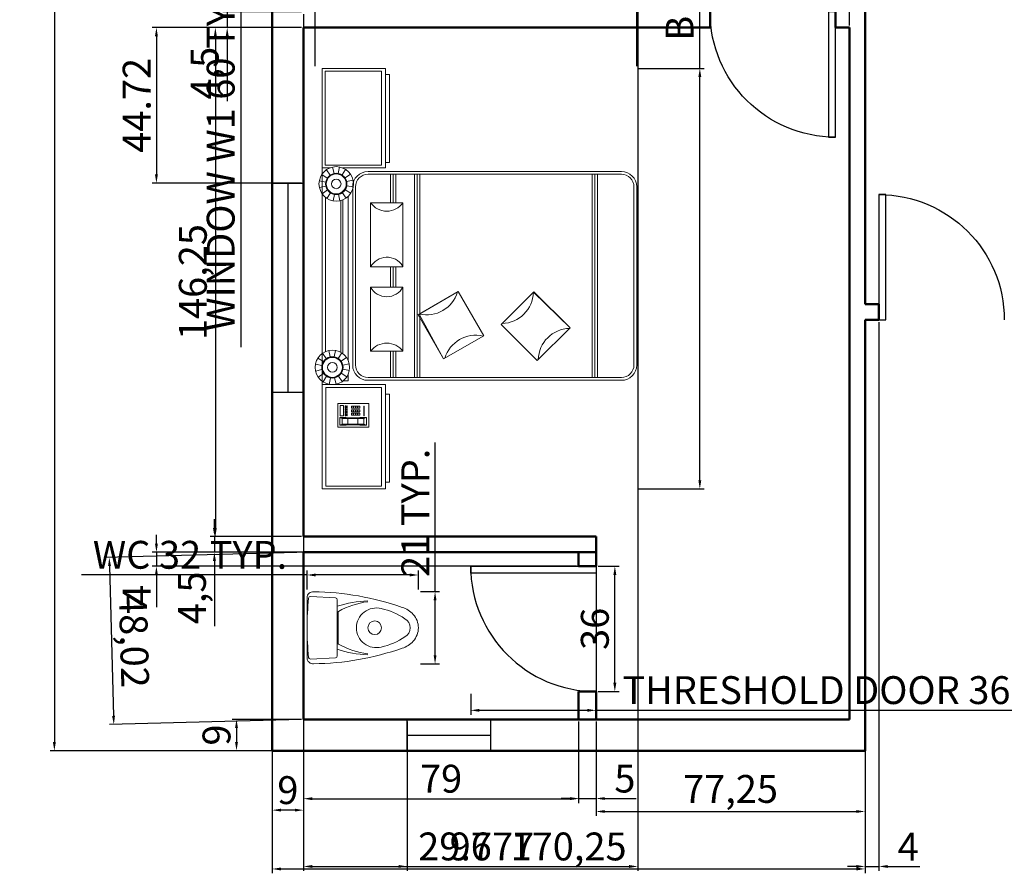
# Model space of a CAD drawing. Units: inches. Extents: x -349 to 9053, y 635 to 6001.
# Tile 2 of 7: x 257 to 540, y 635 to 880. Entities that reach past the tile are written whole.
import ezdxf

# ---------------------------------------------------------------- set-up
doc = ezdxf.new("R2010")
doc.units = ezdxf.units.IN
for name, color, linetype, lineweight in [('A-ANNO-DIMS', 2, 'Continuous', 18), ('A-DOOR', 3, 'Continuous', 25), ('A-FLOR-FIXT', 7, 'Continuous', 18), ('A-FURN', 8, 'Continuous', 18), ('A-GLAZ', 4, 'Continuous', 25), ('A-WALL', 7, 'Continuous', 50)]:
    doc.layers.add(name, color=color, linetype=linetype, lineweight=lineweight)
doc.styles.get("Standard").update_dxf_attribs({"font": 'arial.ttf'})
doc.dimstyles.new('ISO-25', dxfattribs={"dimtxt": 8, "dimasz": 2.5, "dimexe": 1.25, "dimexo": 0.625, "dimtad": 1, "dimtxsty": 'Standard', "dimcen": 2.5, "dimadec": 0, "dimazin": 0, "dimtfac": 1, "dimtmove": 0, "dimatfit": 3, "dimfxl": 1, "dimarcsym": 0})

# ---------------------------------------------------------------- blocks, each defined once
blk = doc.blocks.new('A$C18EB7ED0')
for p, q in [((0.7653, 2.1814), (0.7911, 2.1442)), ((0.8076, 2.1998), (0.8172, 2.1555)), ((0.8537, 2.2006), (0.8456, 2.1559)), ((0.8966, 2.1836), (0.8721, 2.1455)), ((2.0643, 2.1733), (2.0739, 2.129)), ((2.1105, 2.1741), (2.1024, 2.1295)), ((0, 2.1539), (2.8801, 2.1539)), ((0, 1.7209), (0, 2.1539)), ((0.0187, 2.129), (0.695, 2.129)), ((0.0187, 1.7489), (0.0187, 2.129)), ((0.695, 2.129), (0.695, 1.7489)), ((0.7156, 2.1539), (0.7156, 1.7209)), ((0.7162, 2.1054), (0.7608, 2.0973)), ((0.7332, 2.1483), (0.7713, 2.1237)), ((0.9298, 2.1515), (0.8925, 2.1257)), ((0.9481, 2.1092), (0.9038, 2.0996)), ((0.941, 2.1314), (1.9968, 2.1314)), ((1.9899, 2.1218), (2.028, 2.0973)), ((2.022, 2.155), (2.0478, 2.1177)), ((2.1534, 2.1571), (2.1288, 2.119)), ((2.1865, 2.1251), (2.1493, 2.0992)), ((2.1997, 2.1), (2.1997, 2.1539)), ((2.2184, 2.1337), (2.8624, 2.1337)), ((2.2184, 1.7489), (2.2184, 2.1337)), ((2.8624, 2.1337), (2.8624, 1.7489)), ((2.8801, 2.1539), (2.8801, 1.7209)), ((0.5857, 2.0461), (0.4227, 2.0461)), ((0.4227, 2.0461), (0.4227, 1.8353)), ((0.4366, 2.0335), (0.4439, 2.018)), ((0.4903, 2.0335), (0.4366, 2.0335)), ((0.4366, 2.0335), (0.4366, 1.9902)), ((0.4824, 2.018), (0.4903, 2.0335)), ((0.4903, 1.9902), (0.4903, 2.0338)), ((0.5706, 2.0307), (0.4996, 2.0307)), ((0.4996, 2.0307), (0.4996, 2.0082)), ((0.5706, 2.0082), (0.5706, 2.0307)), ((0.5857, 1.8353), (0.5857, 2.0461)), ((0.717, 2.0593), (0.7613, 2.0688)), ((0.7353, 2.0169), (0.7726, 2.0427)), ((0.7685, 1.9849), (0.7931, 2.023)), ((0.8999, 1.987), (0.8741, 2.0243)), ((0.9319, 2.0202), (0.8938, 2.0447)), ((0.9489, 2.0631), (0.9043, 2.0712)), ((1.9752, 2.0268), (0.9359, 2.0268)), ((1.973, 2.0789), (2.0176, 2.0708)), ((1.9737, 2.0328), (2.0181, 2.0424)), ((2.2049, 2.0827), (2.1606, 2.0731)), ((2.2056, 2.0366), (2.161, 2.0447)), ((0.4366, 1.9902), (0.4391, 1.9789)), ((0.4391, 1.9789), (0.4391, 1.9067)), ((0.4824, 2.018), (0.4439, 2.018)), ((0.4824, 2.018), (0.4439, 2.018)), ((0.4439, 2.018), (0.4439, 1.8697)), ((0.4824, 1.978), (0.4439, 1.978)), ((0.4824, 1.8697), (0.4824, 2.018)), ((0.4903, 1.9902), (0.4871, 1.9789)), ((0.4871, 1.9789), (0.4871, 1.908)), ((0.4996, 2.0082), (0.5706, 2.0082)), ((0.514, 1.9963), (0.5013, 1.9963)), ((0.5013, 1.9963), (0.5013, 1.992)), ((0.5013, 1.992), (0.514, 1.992)), ((0.514, 1.9864), (0.5013, 1.9864)), ((0.5013, 1.9864), (0.5013, 1.9821)), ((0.5013, 1.9821), (0.514, 1.9821)), ((0.514, 1.992), (0.514, 1.9963)), ((0.514, 1.9821), (0.514, 1.9864)), ((0.5324, 1.9963), (0.5196, 1.9963)), ((0.5196, 1.9963), (0.5196, 1.992)), ((0.5196, 1.992), (0.5324, 1.992)), ((0.5324, 1.9864), (0.5196, 1.9864)), ((0.5196, 1.9864), (0.5196, 1.9821)), ((0.5196, 1.9821), (0.5324, 1.9821)), ((0.5324, 1.992), (0.5324, 1.9963)), ((0.5324, 1.9821), (0.5324, 1.9864)), ((0.5507, 1.9963), (0.538, 1.9963)), ((0.538, 1.9963), (0.538, 1.992)), ((0.538, 1.992), (0.5507, 1.992)), ((0.5507, 1.9864), (0.538, 1.9864)), ((0.538, 1.9864), (0.538, 1.9821)), ((0.538, 1.9821), (0.5507, 1.9821)), ((0.5507, 1.992), (0.5507, 1.9963)), ((0.5507, 1.9821), (0.5507, 1.9864)), ((0.5691, 1.9963), (0.5564, 1.9963)), ((0.5564, 1.9963), (0.5564, 1.992)), ((0.5564, 1.992), (0.5691, 1.992)), ((0.5691, 1.9864), (0.5564, 1.9864)), ((0.5564, 1.9864), (0.5564, 1.9821)), ((0.5564, 1.9821), (0.5691, 1.9821)), ((0.5691, 1.992), (0.5691, 1.9963)), ((0.5691, 1.9821), (0.5691, 1.9864)), ((0.7411, 2.0132), (0.7411, 1.9754)), ((0.7411, 1.9754), (0.7863, 1.9754)), ((0.8114, 1.9679), (0.8195, 2.0125)), ((0.8575, 1.9687), (0.848, 2.013)), ((0.8788, 1.9754), (2.0045, 1.9754)), ((1.9798, 2.0132), (0.9271, 2.0132)), ((1.9921, 1.9905), (2.0294, 2.0163)), ((2.0252, 1.9584), (2.0498, 1.9965)), ((2.0682, 1.9414), (2.0763, 1.986)), ((2.1143, 1.9422), (2.1047, 1.9865)), ((2.1566, 1.9605), (2.1308, 1.9978)), ((2.1887, 1.9937), (2.1506, 2.0183)), ((2.1742, 1.9754), (2.1771, 1.9754)), ((2.1771, 1.9754), (2.1771, 1.9785)), ((2.1997, 1.7209), (2.1997, 2.0155)), ((0.4391, 1.9067), (0.4366, 1.8971)), ((0.4366, 1.8971), (0.4366, 1.8504)), ((0.4439, 1.9101), (0.4824, 1.9101)), ((0.4871, 1.908), (0.4903, 1.8971)), ((0.4903, 1.8499), (0.4903, 1.8971)), ((0.52, 1.9534), (0.5062, 1.9534)), ((0.5062, 1.9534), (0.5062, 1.9417)), ((0.5062, 1.9417), (0.52, 1.9417)), ((0.52, 1.9385), (0.5062, 1.9385)), ((0.5062, 1.9385), (0.5062, 1.9269)), ((0.5062, 1.9269), (0.52, 1.9269)), ((0.52, 1.9237), (0.5062, 1.9237)), ((0.5062, 1.9237), (0.5062, 1.9121)), ((0.5062, 1.9121), (0.52, 1.9121)), ((0.52, 1.9089), (0.5062, 1.9089)), ((0.5062, 1.9089), (0.5062, 1.8972)), ((0.5062, 1.8972), (0.52, 1.8972)), ((0.52, 1.9417), (0.52, 1.9534)), ((0.52, 1.9269), (0.52, 1.9385)), ((0.52, 1.9121), (0.52, 1.9237)), ((0.52, 1.8972), (0.52, 1.9089)), ((0.5426, 1.9534), (0.5288, 1.9534)), ((0.5288, 1.9534), (0.5288, 1.9417)), ((0.5288, 1.9417), (0.5426, 1.9417)), ((0.5426, 1.9385), (0.5288, 1.9385)), ((0.5288, 1.9385), (0.5288, 1.9269)), ((0.5288, 1.9269), (0.5426, 1.9269)), ((0.5426, 1.9237), (0.5288, 1.9237)), ((0.5288, 1.9237), (0.5288, 1.9121)), ((0.5288, 1.9121), (0.5426, 1.9121)), ((0.5426, 1.9089), (0.5288, 1.9089)), ((0.5288, 1.9089), (0.5288, 1.8972)), ((0.5288, 1.8972), (0.5426, 1.8972)), ((0.5426, 1.9417), (0.5426, 1.9534)), ((0.5426, 1.9269), (0.5426, 1.9385)), ((0.5426, 1.9121), (0.5426, 1.9237)), ((0.5426, 1.8972), (0.5426, 1.9089)), ((0.5659, 1.9534), (0.5521, 1.9534)), ((0.5521, 1.9534), (0.5521, 1.9417)), ((0.5521, 1.9417), (0.5659, 1.9417)), ((0.5659, 1.9385), (0.5521, 1.9385)), ((0.5521, 1.9385), (0.5521, 1.9269)), ((0.5521, 1.9269), (0.5659, 1.9269)), ((0.5659, 1.9237), (0.5521, 1.9237)), ((0.5521, 1.9237), (0.5521, 1.9121)), ((0.5521, 1.9121), (0.5659, 1.9121)), ((0.5659, 1.9089), (0.5521, 1.9089)), ((0.5521, 1.9089), (0.5521, 1.8972)), ((0.5521, 1.8972), (0.5659, 1.8972)), ((0.5659, 1.9417), (0.5659, 1.9534)), ((0.5659, 1.9269), (0.5659, 1.9385)), ((0.5659, 1.9121), (0.5659, 1.9237)), ((0.5659, 1.8972), (0.5659, 1.9089)), ((2.0691, 1.9452), (0.8491, 1.9452)), ((2.0691, 1.926), (0.8491, 1.926)), ((0.4227, 1.8353), (0.5857, 1.8353)), ((0.4439, 1.8697), (0.4366, 1.8504)), ((0.4366, 1.8504), (0.4903, 1.8504)), ((0.4824, 1.8697), (0.4439, 1.8697)), ((0.4439, 1.8697), (0.4824, 1.8697)), ((0.4903, 1.8504), (0.4824, 1.8697)), ((0.5208, 1.8697), (0.5009, 1.8697)), ((0.5009, 1.8697), (0.5009, 1.8657)), ((0.5009, 1.8657), (0.5208, 1.8657)), ((0.5208, 1.8657), (0.5208, 1.8697)), ((0.5433, 1.8697), (0.5234, 1.8697)), ((0.5234, 1.8697), (0.5234, 1.8657)), ((0.5234, 1.8657), (0.5433, 1.8657)), ((0.5433, 1.8657), (0.5433, 1.8697)), ((0.5658, 1.8697), (0.546, 1.8697)), ((0.546, 1.8697), (0.546, 1.8657)), ((0.546, 1.8657), (0.5658, 1.8657)), ((0.5658, 1.8657), (0.5658, 1.8697)), ((0.7439, 1.8401), (0.7439, 0.1052)), ((0.7632, 1.8401), (0.7632, 0.1052)), ((0.9429, 1.8231), (1.3829, 1.8231)), ((0.9429, 1.601), (0.9429, 1.8231)), ((1.3829, 1.8231), (1.3829, 1.601)), ((1.5207, 1.601), (1.5207, 1.8231)), ((1.5207, 1.8231), (1.9608, 1.8231)), ((1.9608, 1.8231), (1.9608, 1.601)), ((2.155, 0.1052), (2.155, 1.8401)), ((2.1743, 0.1052), (2.1743, 1.8401)), ((0.7156, 1.7209), (0, 1.7209)), ((0, 1.7209), (0.6483, 1.7209)), ((0.695, 1.7489), (0.0187, 1.7489)), ((0.0462, 1.6929), (0.0462, 1.7209)), ((0.6483, 1.6929), (0.0462, 1.6929)), ((0.6483, 1.7209), (0.6483, 1.6929)), ((0.7632, 1.6858), (0.9429, 1.6858)), ((1.3829, 1.6858), (1.5207, 1.6858)), ((1.9608, 1.6858), (2.155, 1.6858)), ((2.8801, 1.7209), (2.1997, 1.7209)), ((2.8624, 1.7489), (2.2184, 1.7489)), ((2.2369, 1.7209), (2.8801, 1.7209)), ((2.2369, 1.6929), (2.2369, 1.7209)), ((2.839, 1.6929), (2.2369, 1.6929)), ((2.839, 1.7209), (2.839, 1.6929)), ((0.7632, 1.6678), (0.9429, 1.6678)), ((0.7632, 1.6498), (0.9429, 1.6498)), ((1.3829, 1.6678), (1.5207, 1.6678)), ((1.3829, 1.6498), (1.5207, 1.6498)), ((1.9608, 1.6678), (2.155, 1.6678)), ((1.9608, 1.6498), (2.155, 1.6498)), ((1.3829, 1.601), (0.9429, 1.601)), ((1.9608, 1.601), (1.5207, 1.601)), ((0.7632, 1.5215), (2.155, 1.5215)), ((0.7632, 1.5035), (2.155, 1.5035)), ((0.7632, 1.4855), (2.155, 1.4855)), ((0.8904, 1.3226), (1.1935, 1.4976)), ((0.8904, 1.3226), (1.1982, 1.4894)), ((1.1935, 1.4976), (1.3524, 1.2224)), ((1.1982, 1.4894), (1.3524, 1.2224)), ((1.0493, 1.0474), (0.8904, 1.3226)), ((1.0493, 1.0474), (0.8904, 1.3226)), ((1.3524, 1.2224), (1.0493, 1.0474)), ((1.3524, 1.2224), (1.0493, 1.0474)), ((0.8789, 0.6811), (1.1264, 0.9286)), ((0.8789, 0.6811), (1.1264, 0.9286)), ((1.1264, 0.9286), (1.3473, 0.7077)), ((1.1264, 0.9286), (1.3511, 0.7039)), ((1.1036, 0.4564), (0.8789, 0.6811)), ((1.1036, 0.4564), (0.8789, 0.6811)), ((1.3473, 0.7077), (1.1036, 0.4564)), ((1.3511, 0.7039), (1.1036, 0.4564)), ((0.7632, 0.3045), (2.155, 0.3045)), ((0.7632, 0.2865), (2.155, 0.2865)), ((0.7632, 0.2685), (2.155, 0.2685)), ((0.8491, 0.0193), (2.0691, 0.0193)), ((0.8491, 0), (2.0691, 0))]:
    blk.add_line(p, q)
for centre, radius in [((0.8326, 2.0842), 0.1182), ((2.0893, 2.0578), 0.1182), ((0.8326, 2.0842), 0.0729), ((0.8326, 2.0842), 0.0684), ((0.8326, 2.0842), 0.0328), ((2.0893, 2.0578), 0.0729), ((2.0893, 2.0578), 0.0684), ((2.0893, 2.0578), 0.0328)]:
    blk.add_circle(centre, radius)
for centre, radius, start, end in [((0.8491, 1.8401), 0.1052, 90, 180), ((0.8491, 1.8401), 0.0859, 90, 180), ((2.0691, 1.8401), 0.1052, 0, 90), ((2.0691, 1.8401), 0.0859, 0, 90), ((0.8604, 1.712), 0.1383, 306.59595, 53.40405), ((1.4431, 1.712), 0.1263, 118.46186, 241.53814), ((1.4584, 1.7106), 0.1286, 303.40233, 61.02638), ((2.0371, 1.712), 0.1347, 124.50267, 235.49733), ((1.4126, 1.4383), 0.2204, 166.58792, 253.41208), ((0.8322, 1.1031), 0.2204, 346.58792, 73.41208), ((1.3534, 0.928), 0.2204, 181.58792, 268.41208), ((0.8795, 0.4541), 0.2204, 1.58792, 88.41208), ((0.8491, 0.1052), 0.1052, 180, 270), ((0.8491, 0.1052), 0.0859, 180, 270), ((2.0691, 0.1052), 0.1052, 270, 0), ((2.0691, 0.1052), 0.0859, 270, 0)]:
    blk.add_arc(centre, radius, start, end)
blk = doc.blocks.new('A$C444A5E9C')
at = {"ltscale": 20}
for p, q in [((0.2458, 0.76), (0.0398, 0.76)), ((0.0411, 0.5655), (0.0321, 0.7371)), ((0.0536, 0.5537), (0.2458, 0.5537)), ((0.141, 0.5487), (0.2458, 0.5487))]:
    blk.add_line(p, q, dxfattribs=at)
for p, q in [((0.2458, 0.76), (0.4517, 0.76)), ((0.4504, 0.5655), (0.4594, 0.7371)), ((0.4379, 0.5537), (0.2458, 0.5537)), ((0.3505, 0.5487), (0.2458, 0.5487))]:
    blk.add_line(p, q)
blk.add_circle((0.2458, 0.2982), 0.0465, dxfattribs=at)
for centre, radius, start, end in [((0.0398, 0.72), 0.04, 90, 185.821), ((0.0441, 0.7377), 0.012, 95.84387, 183), ((0.2455, -1.2297), 1.9897, 89.99241, 95.84387), ((1.8697, 0.7335), 1.8698, 180.53729, 199.44062), ((0.0536, 0.5662), 0.0125, 183, 270), ((0.7661, 0.3277), 0.7045, 161.29061, 178.53633), ((0.58, 0.2848), 0.5159, 149.71646, 173.22437), ((0.141, 0.5412), 0.0075, 90, 149.71646), ((0.2463, 0.2875), 0.1361, 90.23685, 194.54903), ((0.2452, 0.2875), 0.1361, 345.45097, 89.76315), ((0.561, 0.3494), 0.4566, 192.1399, 214.27057), ((-0.0695, 0.3494), 0.4566, 325.72943, 347.8601), ((0.2665, 0.1585), 0.1669, 196.47232, 227.66237), ((0.2465, 0.1287), 0.0727, 210.08399, 269.41891), ((0.245, 0.1287), 0.0727, 270.58109, 329.91601), ((0.2458, 0.137), 0.137, 228.04012, 270)]:
    blk.add_arc(centre, radius, start, end, dxfattribs=at)
for centre, radius, start, end in [((0.246, -1.2297), 1.9897, 84.15613, 90.00759), ((0.4474, 0.7377), 0.012, 357, 84.15613), ((0.4517, 0.72), 0.04, 354.179, 90), ((-1.3782, 0.7335), 1.8698, 340.55938, 359.46271), ((0.3505, 0.5412), 0.0075, 30.28354, 90), ((-0.0885, 0.2848), 0.5159, 6.77563, 30.28354), ((-0.2746, 0.3277), 0.7045, 1.46367, 18.70939), ((0.4379, 0.5662), 0.0125, 270, 357), ((0.225, 0.1585), 0.1669, 312.33763, 343.52768), ((0.2458, 0.137), 0.137, 270, 311.95988)]:
    blk.add_arc(centre, radius, start, end)
blk = doc.blocks.new('*D20')
at = {"layer": 'A-ANNO-DIMS', "color": 0, "lineweight": -2, "transparency": 16777216}
for p, q in [((317.08, 884.75), (317.08, 887.25)), ((338.38, 882.25), (315.83, 882.25)), ((317.08, 882.25), (317.08, 877.75)), ((338.38, 877.75), (315.83, 877.75)), ((317.08, 875.25), (317.08, 856.55))]:
    blk.add_line(p, q, dxfattribs=at)
at = {"layer": 'A-ANNO-DIMS', "color": 0, "transparency": 16777216}
for points in [[(316.66, 884.75), (317.5, 884.75), (317.08, 882.25)], [(316.66, 875.25), (317.5, 875.25), (317.08, 877.75)]]:
    blk.add_solid(points, dxfattribs=at)
at = {"layer": 'Defpoints', "color": 0, "transparency": 16777216}
for p in [(339, 882.25), (317.08, 877.75), (339, 877.75)]:
    blk.add_point(p, dxfattribs=at)
at = {"layer": 'A-ANNO-DIMS', "color": 0, "transparency": 16777216, "insert": (311.66, 864.65), "char_height": 8, "attachment_point": 5, "rotation": 90}
blk.add_mtext('4,5', dxfattribs=at)
blk = doc.blocks.new('*D21')
at = {"layer": 'A-ANNO-DIMS', "color": 0, "lineweight": -2, "transparency": 16777216}
for p, q in [((338.38, 877.75), (312.42, 877.75)), ((313.67, 875.25), (313.67, 734)), ((338.38, 731.5), (312.42, 731.5))]:
    blk.add_line(p, q, dxfattribs=at)
at = {"layer": 'A-ANNO-DIMS', "color": 0, "transparency": 16777216}
for points in [[(313.26, 875.25), (314.09, 875.25), (313.67, 877.75)], [(313.26, 734), (314.09, 734), (313.67, 731.5)]]:
    blk.add_solid(points, dxfattribs=at)
at = {"layer": 'Defpoints', "color": 0, "transparency": 16777216}
for p in [(339, 877.75), (313.67, 731.5), (339, 731.5)]:
    blk.add_point(p, dxfattribs=at)
at = {"layer": 'A-ANNO-DIMS', "color": 0, "transparency": 16777216, "insert": (308.24, 804.62), "char_height": 8, "attachment_point": 5, "rotation": 90}
blk.add_mtext('146,25', dxfattribs=at)
blk = doc.blocks.new('*D22')
at = {"layer": 'A-ANNO-DIMS', "color": 0, "lineweight": -2, "transparency": 16777216}
for p, q in [((313.4, 734), (313.4, 736.5)), ((338.38, 731.5), (312.15, 731.5)), ((313.4, 731.5), (313.4, 727)), ((338.38, 727), (312.15, 727)), ((313.4, 724.5), (313.4, 705.8))]:
    blk.add_line(p, q, dxfattribs=at)
at = {"layer": 'A-ANNO-DIMS', "color": 0, "transparency": 16777216}
for points in [[(312.99, 734), (313.82, 734), (313.4, 731.5)], [(312.99, 724.5), (313.82, 724.5), (313.4, 727)]]:
    blk.add_solid(points, dxfattribs=at)
at = {"layer": 'Defpoints', "color": 0, "transparency": 16777216}
for p in [(339, 731.5), (313.4, 727), (339, 727)]:
    blk.add_point(p, dxfattribs=at)
at = {"layer": 'A-ANNO-DIMS', "color": 0, "transparency": 16777216, "insert": (307.99, 713.9), "char_height": 8, "attachment_point": 5, "rotation": 90}
blk.add_mtext('4,5', dxfattribs=at)
blk = doc.blocks.new('*D23')
at = {"layer": 'A-ANNO-DIMS', "color": 0, "lineweight": -2, "transparency": 16777216}
for p, q in [((337.08, 726.98), (281.96, 725.49)), ((283.28, 723.03), (284.44, 680.02)), ((338.38, 678.98), (283.26, 677.49))]:
    blk.add_line(p, q, dxfattribs=at)
at = {"layer": 'A-ANNO-DIMS', "color": 0, "transparency": 16777216}
for points in [[(283.69, 723.04), (282.86, 723.02), (283.21, 725.53)], [(284.86, 680.04), (284.02, 680.01), (284.51, 677.53)]]:
    blk.add_solid(points, dxfattribs=at)
at = {"layer": 'Defpoints', "color": 0, "transparency": 16777216}
for p in [(337.7, 727), (339, 679), (284.51, 677.53)]:
    blk.add_point(p, dxfattribs=at)
at = {"layer": 'A-ANNO-DIMS', "color": 0, "transparency": 16777216, "insert": (289.29, 701.67), "char_height": 8, "attachment_point": 5, "rotation": 271.5498}
blk.add_mtext('48,02', dxfattribs=at)
blk = doc.blocks.new('*D24')
at = {"layer": 'A-ANNO-DIMS', "color": 0, "lineweight": -2, "transparency": 16777216}
for p, q in [((338.38, 679), (318.49, 679)), ((319.74, 676.5), (319.74, 672.5)), ((338.38, 670), (318.49, 670))]:
    blk.add_line(p, q, dxfattribs=at)
at = {"layer": 'A-ANNO-DIMS', "color": 0, "transparency": 16777216}
for points in [[(319.33, 676.5), (320.16, 676.5), (319.74, 679)], [(319.33, 672.5), (320.16, 672.5), (319.74, 670)]]:
    blk.add_solid(points, dxfattribs=at)
at = {"layer": 'Defpoints', "color": 0, "transparency": 16777216}
for p in [(339, 679), (319.74, 670), (339, 670)]:
    blk.add_point(p, dxfattribs=at)
at = {"layer": 'A-ANNO-DIMS', "color": 0, "transparency": 16777216, "insert": (315.04, 674.5), "char_height": 8, "attachment_point": 5, "rotation": 90}
blk.add_mtext('9', dxfattribs=at)
blk = doc.blocks.new('*D25')
at = {"layer": 'A-ANNO-DIMS', "color": 0, "lineweight": -2, "transparency": 16777216}
for p, q in [((330, 678.38), (330, 651.68)), ((339, 678.38), (339, 651.68)), ((336.5, 652.93), (332.5, 652.93))]:
    blk.add_line(p, q, dxfattribs=at)
at = {"layer": 'A-ANNO-DIMS', "color": 0, "transparency": 16777216}
for points in [[(332.5, 653.35), (332.5, 652.52), (330, 652.93)], [(336.5, 653.35), (336.5, 652.52), (339, 652.93)]]:
    blk.add_solid(points, dxfattribs=at)
at = {"layer": 'Defpoints', "color": 0, "transparency": 16777216}
for p in [(330, 679), (339, 679), (330, 652.93)]:
    blk.add_point(p, dxfattribs=at)
at = {"layer": 'A-ANNO-DIMS', "color": 0, "transparency": 16777216, "insert": (334.5, 657.64), "char_height": 8, "attachment_point": 5}
blk.add_mtext('9', dxfattribs=at)
blk = doc.blocks.new('*D26')
at = {"layer": 'A-ANNO-DIMS', "color": 0, "lineweight": -2, "transparency": 16777216}
for p, q in [((339, 678.38), (339, 654.96)), ((418, 678.38), (418, 654.96)), ((341.5, 656.21), (415.5, 656.21))]:
    blk.add_line(p, q, dxfattribs=at)
at = {"layer": 'A-ANNO-DIMS', "color": 0, "transparency": 16777216}
for points in [[(341.5, 656.63), (341.5, 655.8), (339, 656.21)], [(415.5, 656.63), (415.5, 655.8), (418, 656.21)]]:
    blk.add_solid(points, dxfattribs=at)
at = {"layer": 'Defpoints', "color": 0, "transparency": 16777216}
for p in [(339, 679), (418, 679), (418, 656.21)]:
    blk.add_point(p, dxfattribs=at)
at = {"layer": 'A-ANNO-DIMS', "color": 0, "transparency": 16777216, "insert": (378.5, 660.92), "char_height": 8, "attachment_point": 5}
blk.add_mtext('79', dxfattribs=at)
blk = doc.blocks.new('*D27')
at = {"layer": 'A-ANNO-DIMS', "color": 0, "lineweight": -2, "transparency": 16777216}
for p, q in [((418, 678.38), (418, 655.02)), ((423, 678.38), (423, 655.02)), ((415.5, 656.27), (413, 656.27)), ((418, 656.27), (423, 656.27)), ((425.5, 656.27), (434.55, 656.27))]:
    blk.add_line(p, q, dxfattribs=at)
at = {"layer": 'A-ANNO-DIMS', "color": 0, "transparency": 16777216}
for points in [[(415.5, 656.68), (415.5, 655.85), (418, 656.27)], [(425.5, 656.68), (425.5, 655.85), (423, 656.27)]]:
    blk.add_solid(points, dxfattribs=at)
at = {"layer": 'Defpoints', "color": 0, "transparency": 16777216}
for p in [(418, 679), (423, 679), (423, 656.27)]:
    blk.add_point(p, dxfattribs=at)
at = {"layer": 'A-ANNO-DIMS', "color": 0, "transparency": 16777216, "insert": (431.28, 660.96), "char_height": 8, "attachment_point": 5}
blk.add_mtext('5', dxfattribs=at)
blk = doc.blocks.new('*D28')
at = {"layer": 'A-ANNO-DIMS', "color": 0, "lineweight": -2, "transparency": 16777216}
for p, q in [((423, 678.38), (423, 651.29)), ((500.25, 678.38), (500.25, 651.29)), ((425.5, 652.54), (497.75, 652.54))]:
    blk.add_line(p, q, dxfattribs=at)
at = {"layer": 'A-ANNO-DIMS', "color": 0, "transparency": 16777216}
for points in [[(425.5, 652.96), (425.5, 652.13), (423, 652.54)], [(497.75, 652.96), (497.75, 652.13), (500.25, 652.54)]]:
    blk.add_solid(points, dxfattribs=at)
at = {"layer": 'Defpoints', "color": 0, "transparency": 16777216}
for p in [(423, 679), (500.25, 679), (500.25, 652.54)]:
    blk.add_point(p, dxfattribs=at)
at = {"layer": 'A-ANNO-DIMS', "color": 0, "transparency": 16777216, "insert": (461.62, 657.98), "char_height": 8, "attachment_point": 5}
blk.add_mtext('77,25', dxfattribs=at)
blk = doc.blocks.new('*D29')
at = {"layer": 'A-ANNO-DIMS', "color": 0, "lineweight": -2, "transparency": 16777216}
for p, q in [((330, 669.38), (330, 634.78)), ((500.25, 669.38), (500.25, 634.78)), ((332.5, 636.03), (497.75, 636.03))]:
    blk.add_line(p, q, dxfattribs=at)
at = {"layer": 'A-ANNO-DIMS', "color": 0, "transparency": 16777216}
for points in [[(332.5, 636.45), (332.5, 635.61), (330, 636.03)], [(497.75, 636.45), (497.75, 635.61), (500.25, 636.03)]]:
    blk.add_solid(points, dxfattribs=at)
at = {"layer": 'Defpoints', "color": 0, "transparency": 16777216}
for p in [(330, 670), (500.25, 670), (500.25, 636.03)]:
    blk.add_point(p, dxfattribs=at)
at = {"layer": 'A-ANNO-DIMS', "color": 0, "transparency": 16777216, "insert": (415.12, 641.46), "char_height": 8, "attachment_point": 5}
blk.add_mtext('170,25', dxfattribs=at)
blk = doc.blocks.new('*D31')
at = {"layer": 'A-ANNO-DIMS', "color": 0, "lineweight": -2, "transparency": 16777216}
for p, q in [((338.38, 1126), (266.19, 1126)), ((267.44, 1123.5), (267.44, 672.5)), ((338.38, 670), (266.19, 670))]:
    blk.add_line(p, q, dxfattribs=at)
at = {"layer": 'A-ANNO-DIMS', "color": 0, "transparency": 16777216}
for points in [[(267.02, 1123.5), (267.86, 1123.5), (267.44, 1126)], [(267.02, 672.5), (267.86, 672.5), (267.44, 670)]]:
    blk.add_solid(points, dxfattribs=at)
at = {"layer": 'Defpoints', "color": 0, "transparency": 16777216}
for p in [(339, 1126), (267.44, 670), (339, 670)]:
    blk.add_point(p, dxfattribs=at)
at = {"layer": 'A-ANNO-DIMS', "color": 0, "transparency": 16777216, "insert": (262.73, 898), "char_height": 8, "attachment_point": 5, "rotation": 90}
blk.add_mtext('456', dxfattribs=at)
blk = doc.blocks.new('DOOR-36IN-SWING-WITH-THRESHOLD')
blk.add_line((0, 0), (0, -36))
blk.add_lwpolyline([(-36, 0), (0, 0), (0, -2), (-36, -2)], close=True)
blk.add_arc((0, 0), 36, 180, 270)
blk = doc.blocks.new('DOOR-36IN-SWING')
blk.add_line((0, 0), (-2, 0))
blk.add_lwpolyline([(0, 36), (0, 0), (-2, 0), (-2, 36)], close=True)
blk.add_arc((0, 0), 36, 90, 180)
blk = doc.blocks.new('WIN-60IN')
for p, q in [((0, -4.5), (0, 4.5)), ((60, -4.5), (60, 4.5)), ((0, 0), (60, 0))]:
    blk.add_line(p, q)
blk = doc.blocks.new('WIN-24IN')
for p, q in [((0, -4.5), (0, 4.5)), ((24, -4.5), (24, 4.5)), ((0, 0), (24, 0))]:
    blk.add_line(p, q)
blk = doc.blocks.new('*D41')
at = {"layer": 'A-ANNO-DIMS', "color": 0, "lineweight": -2, "transparency": 16777216}
for p, q in [((387, 686.37), (387, 680.35)), ((423, 686.37), (423, 680.35)), ((389.5, 681.6), (420.5, 681.6)), ((423, 681.6), (547.07, 681.6))]:
    blk.add_line(p, q, dxfattribs=at)
at = {"layer": 'A-ANNO-DIMS', "color": 0, "transparency": 16777216}
for points in [[(389.5, 682.02), (389.5, 681.18), (387, 681.6)], [(420.5, 682.02), (420.5, 681.18), (423, 681.6)]]:
    blk.add_solid(points, dxfattribs=at)
at = {"layer": 'Defpoints', "color": 0, "transparency": 16777216}
for p in [(387, 687), (423, 687), (423, 681.6)]:
    blk.add_point(p, dxfattribs=at)
at = {"layer": 'A-ANNO-DIMS', "color": 0, "transparency": 16777216, "insert": (486.29, 686.37), "char_height": 8, "attachment_point": 5}
blk.add_mtext('THRESHOLD DOOR 36', dxfattribs=at)
blk = doc.blocks.new('*D42')
at = {"layer": 'A-ANNO-DIMS', "color": 0, "lineweight": -2, "transparency": 16777216}
for p, q in [((423.63, 723), (429.65, 723)), ((428.4, 689.5), (428.4, 720.5)), ((423.63, 687), (429.65, 687))]:
    blk.add_line(p, q, dxfattribs=at)
at = {"layer": 'A-ANNO-DIMS', "color": 0, "transparency": 16777216}
for points in [[(427.98, 720.5), (428.82, 720.5), (428.4, 723)], [(427.98, 689.5), (428.82, 689.5), (428.4, 687)]]:
    blk.add_solid(points, dxfattribs=at)
at = {"layer": 'Defpoints', "color": 0, "transparency": 16777216}
for p in [(423, 723), (428.4, 723), (423, 687)]:
    blk.add_point(p, dxfattribs=at)
at = {"layer": 'A-ANNO-DIMS', "color": 0, "transparency": 16777216, "insert": (423.69, 705), "char_height": 8, "attachment_point": 5, "rotation": 90}
blk.add_mtext('36', dxfattribs=at)
blk = doc.blocks.new('*D45')
at = {"layer": 'A-ANNO-DIMS', "color": 0, "lineweight": -2, "transparency": 16777216}
for p, q in [((329.38, 961), (319.75, 961)), ((321, 958.5), (321, 903.5)), ((329.38, 901), (319.75, 901)), ((321, 901), (321, 785.97))]:
    blk.add_line(p, q, dxfattribs=at)
at = {"layer": 'A-ANNO-DIMS', "color": 0, "transparency": 16777216}
for points in [[(320.58, 958.5), (321.42, 958.5), (321, 961)], [(320.58, 903.5), (321.42, 903.5), (321, 901)]]:
    blk.add_solid(points, dxfattribs=at)
at = {"layer": 'Defpoints', "color": 0, "transparency": 16777216}
for p in [(330, 961), (321, 901), (330, 901)]:
    blk.add_point(p, dxfattribs=at)
at = {"layer": 'A-ANNO-DIMS', "color": 0, "transparency": 16777216, "insert": (316.24, 842.24), "char_height": 8, "attachment_point": 5, "rotation": 90}
blk.add_mtext('WINDOW W1 60 TYP.', dxfattribs=at)
blk = doc.blocks.new('*D49')
at = {"layer": 'A-ANNO-DIMS', "color": 0, "lineweight": -2, "transparency": 16777216}
for p, q in [((452.81, 865.99), (452.81, 995.27)), ((435.32, 865.99), (454.06, 865.99)), ((452.81, 747.7), (452.81, 863.49)), ((435.32, 745.2), (454.06, 745.2))]:
    blk.add_line(p, q, dxfattribs=at)
at = {"layer": 'A-ANNO-DIMS', "color": 0, "transparency": 16777216}
for points in [[(452.39, 863.49), (453.23, 863.49), (452.81, 865.99)], [(452.39, 747.7), (453.23, 747.7), (452.81, 745.2)]]:
    blk.add_solid(points, dxfattribs=at)
at = {"layer": 'Defpoints', "color": 0, "transparency": 16777216}
for p in [(434.69, 865.99), (452.81, 865.99), (434.69, 745.2)]:
    blk.add_point(p, dxfattribs=at)
at = {"layer": 'A-ANNO-DIMS', "color": 0, "transparency": 16777216, "insert": (448.04, 931.88), "char_height": 8, "attachment_point": 5, "rotation": 90}
blk.add_mtext('BED GROUP B 121 TYP.', dxfattribs=at)
blk = doc.blocks.new('*D50')
at = {"layer": 'A-ANNO-DIMS', "color": 0, "lineweight": -2, "transparency": 16777216}
for p, q in [((342.32, 866.61), (342.32, 885.35)), ((434.69, 866.61), (434.69, 885.35)), ((432.19, 884.1), (344.82, 884.1))]:
    blk.add_line(p, q, dxfattribs=at)
at = {"layer": 'A-ANNO-DIMS', "color": 0, "transparency": 16777216}
for points in [[(344.82, 884.52), (344.82, 883.69), (342.32, 884.1)], [(432.19, 884.52), (432.19, 883.69), (434.69, 884.1)]]:
    blk.add_solid(points, dxfattribs=at)
at = {"layer": 'Defpoints', "color": 0, "transparency": 16777216}
for p in [(342.32, 884.1), (342.32, 865.99), (434.69, 865.99)]:
    blk.add_point(p, dxfattribs=at)
at = {"layer": 'A-ANNO-DIMS', "color": 0, "transparency": 16777216, "insert": (388.51, 888.81), "char_height": 8, "attachment_point": 5}
blk.add_mtext('92 TYP.', dxfattribs=at)
blk = doc.blocks.new('*D51')
at = {"layer": 'A-ANNO-DIMS', "color": 0, "lineweight": -2, "transparency": 16777216}
for p, q in [((340.02, 716.31), (340.02, 721.73)), ((371.98, 716.31), (371.98, 721.73)), ((340.02, 720.48), (275.28, 720.48)), ((369.48, 720.48), (342.52, 720.48))]:
    blk.add_line(p, q, dxfattribs=at)
at = {"layer": 'A-ANNO-DIMS', "color": 0, "transparency": 16777216}
for points in [[(342.52, 720.9), (342.52, 720.06), (340.02, 720.48)], [(369.48, 720.9), (369.48, 720.06), (371.98, 720.48)]]:
    blk.add_solid(points, dxfattribs=at)
at = {"layer": 'Defpoints', "color": 0, "transparency": 16777216}
for p in [(340.02, 720.48), (340.02, 715.69), (371.98, 715.69)]:
    blk.add_point(p, dxfattribs=at)
at = {"layer": 'A-ANNO-DIMS', "color": 0, "transparency": 16777216, "insert": (306.4, 725.24), "char_height": 8, "attachment_point": 5}
blk.add_mtext('WC 32 TYP.', dxfattribs=at)
blk = doc.blocks.new('*D52')
at = {"layer": 'A-ANNO-DIMS', "color": 0, "lineweight": -2, "transparency": 16777216}
for p, q in [((376.77, 715.69), (376.77, 758.52)), ((372.6, 715.69), (378.02, 715.69)), ((376.77, 697.43), (376.77, 713.19)), ((372.6, 694.93), (378.02, 694.93))]:
    blk.add_line(p, q, dxfattribs=at)
at = {"layer": 'A-ANNO-DIMS', "color": 0, "transparency": 16777216}
for points in [[(376.36, 713.19), (377.19, 713.19), (376.77, 715.69)], [(376.36, 697.43), (377.19, 697.43), (376.77, 694.93)]]:
    blk.add_solid(points, dxfattribs=at)
at = {"layer": 'Defpoints', "color": 0, "transparency": 16777216}
for p in [(371.98, 715.69), (376.77, 715.69), (371.98, 694.93)]:
    blk.add_point(p, dxfattribs=at)
at = {"layer": 'A-ANNO-DIMS', "color": 0, "transparency": 16777216, "insert": (372.13, 738.35), "char_height": 8, "attachment_point": 5, "rotation": 90}
blk.add_mtext('21 TYP.', dxfattribs=at)
blk = doc.blocks.new('*D59')
at = {"layer": 'A-ANNO-DIMS', "color": 0, "lineweight": -2, "transparency": 16777216}
for p, q in [((435, 905.62), (435, 635.5)), ((339, 881.62), (339, 635.5)), ((341.5, 636.75), (432.5, 636.75))]:
    blk.add_line(p, q, dxfattribs=at)
at = {"layer": 'A-ANNO-DIMS', "color": 0, "transparency": 16777216}
for points in [[(341.5, 637.17), (341.5, 636.33), (339, 636.75)], [(432.5, 637.17), (432.5, 636.33), (435, 636.75)]]:
    blk.add_solid(points, dxfattribs=at)
at = {"layer": 'Defpoints', "color": 0, "transparency": 16777216}
for p in [(435, 906.25), (339, 882.25), (435, 636.75)]:
    blk.add_point(p, dxfattribs=at)
at = {"layer": 'A-ANNO-DIMS', "color": 0, "transparency": 16777216, "insert": (387, 641.46), "char_height": 8, "attachment_point": 5}
blk.add_mtext('96', dxfattribs=at)
blk = doc.blocks.new('*D72')
at = {"layer": 'A-ANNO-DIMS', "color": 0, "lineweight": -2, "transparency": 16777216}
for p, q in [((338.38, 877.75), (295.5, 877.75)), ((296.75, 875.25), (296.75, 835.53)), ((338.38, 833.03), (295.5, 833.03))]:
    blk.add_line(p, q, dxfattribs=at)
at = {"layer": 'A-ANNO-DIMS', "color": 0, "transparency": 16777216}
for points in [[(296.33, 875.25), (297.17, 875.25), (296.75, 877.75)], [(296.33, 835.53), (297.17, 835.53), (296.75, 833.03)]]:
    blk.add_solid(points, dxfattribs=at)
at = {"layer": 'Defpoints', "color": 0, "transparency": 16777216}
for p in [(339, 877.75), (296.75, 833.03), (339, 833.03)]:
    blk.add_point(p, dxfattribs=at)
at = {"layer": 'A-ANNO-DIMS', "color": 0, "transparency": 16777216, "insert": (292.11, 855.39), "char_height": 8, "attachment_point": 5, "rotation": 90}
blk.add_mtext('44.72', dxfattribs=at)
blk = doc.blocks.new('*D74')
at = {"layer": 'A-ANNO-DIMS', "color": 0, "lineweight": -2, "transparency": 16777216}
for p, q in [((339, 678.38), (339, 635.5)), ((368.78, 678.38), (368.78, 635.5)), ((341.5, 636.75), (366.28, 636.75)), ((368.78, 636.75), (405.87, 636.75))]:
    blk.add_line(p, q, dxfattribs=at)
at = {"layer": 'A-ANNO-DIMS', "color": 0, "transparency": 16777216}
for points in [[(341.5, 637.17), (341.5, 636.33), (339, 636.75)], [(366.28, 637.17), (366.28, 636.33), (368.78, 636.75)]]:
    blk.add_solid(points, dxfattribs=at)
at = {"layer": 'Defpoints', "color": 0, "transparency": 16777216}
for p in [(339, 679), (368.78, 679), (368.78, 636.75)]:
    blk.add_point(p, dxfattribs=at)
at = {"layer": 'A-ANNO-DIMS', "color": 0, "transparency": 16777216, "insert": (388.58, 641.46), "char_height": 8, "attachment_point": 5}
blk.add_mtext('29.777', dxfattribs=at)
blk = doc.blocks.new('*D75')
at = {"layer": 'A-ANNO-DIMS', "color": 0, "lineweight": -2, "transparency": 16777216}
for p, q in [((296.75, 729.5), (296.75, 732)), ((417.38, 727), (295.5, 727)), ((296.75, 727), (296.75, 723)), ((417.38, 723), (295.5, 723)), ((296.75, 720.5), (296.75, 711.22))]:
    blk.add_line(p, q, dxfattribs=at)
at = {"layer": 'A-ANNO-DIMS', "color": 0, "transparency": 16777216}
for points in [[(296.33, 729.5), (297.17, 729.5), (296.75, 727)], [(296.33, 720.5), (297.17, 720.5), (296.75, 723)]]:
    blk.add_solid(points, dxfattribs=at)
at = {"layer": 'Defpoints', "color": 0, "transparency": 16777216}
for p in [(418, 727), (296.75, 723), (418, 723)]:
    blk.add_point(p, dxfattribs=at)
at = {"layer": 'A-ANNO-DIMS', "color": 0, "transparency": 16777216, "insert": (292.13, 714.61), "char_height": 8, "attachment_point": 5, "rotation": 90}
blk.add_mtext('4', dxfattribs=at)
blk = doc.blocks.new('*D76')
at = {"layer": 'A-ANNO-DIMS', "color": 0, "lineweight": -2, "transparency": 16777216}
for p, q in [((491.75, 878.37), (491.75, 1160.5)), ((495.75, 878.37), (495.75, 1160.5)), ((489.25, 1159.25), (479.97, 1159.25)), ((495.75, 1159.25), (491.75, 1159.25)), ((498.25, 1159.25), (500.75, 1159.25))]:
    blk.add_line(p, q, dxfattribs=at)
at = {"layer": 'A-ANNO-DIMS', "color": 0, "transparency": 16777216}
for points in [[(489.25, 1159.67), (489.25, 1158.83), (491.75, 1159.25)], [(498.25, 1159.67), (498.25, 1158.83), (495.75, 1159.25)]]:
    blk.add_solid(points, dxfattribs=at)
at = {"layer": 'Defpoints', "color": 0, "transparency": 16777216}
for p in [(491.75, 1159.25), (491.75, 877.75), (495.75, 877.75)]:
    blk.add_point(p, dxfattribs=at)
at = {"layer": 'A-ANNO-DIMS', "color": 0, "transparency": 16777216, "insert": (483.36, 1163.88), "char_height": 8, "attachment_point": 5}
blk.add_mtext('4', dxfattribs=at)
blk = doc.blocks.new('*D77')
at = {"layer": 'A-ANNO-DIMS', "color": 0, "lineweight": -2, "transparency": 16777216}
for p, q in [((500.25, 793.12), (500.25, 635.5)), ((504.25, 793.12), (504.25, 635.5)), ((497.75, 636.75), (495.25, 636.75)), ((500.25, 636.75), (504.25, 636.75)), ((506.75, 636.75), (516.03, 636.75))]:
    blk.add_line(p, q, dxfattribs=at)
at = {"layer": 'A-ANNO-DIMS', "color": 0, "transparency": 16777216}
for points in [[(497.75, 637.17), (497.75, 636.33), (500.25, 636.75)], [(506.75, 637.17), (506.75, 636.33), (504.25, 636.75)]]:
    blk.add_solid(points, dxfattribs=at)
at = {"layer": 'Defpoints', "color": 0, "transparency": 16777216}
for p in [(500.25, 793.75), (504.25, 793.75), (504.25, 636.75)]:
    blk.add_point(p, dxfattribs=at)
at = {"layer": 'A-ANNO-DIMS', "color": 0, "transparency": 16777216, "insert": (512.64, 641.38), "char_height": 8, "attachment_point": 5}
blk.add_mtext('4', dxfattribs=at)

msp = doc.modelspace()

# ---------------------------------------------------------------- linework, layer by layer
at = {"layer": 'A-WALL'}
for p, q in [((330, 1126), (330, 670)), ((455.75, 877.75), (455.75, 882.25)), ((491.75, 877.75), (491.75, 882.25)), ((500.25, 882.25), (500.25, 798.25)), ((339, 877.75), (455.75, 877.75)), ((339, 877.75), (339, 731.5)), ((339, 731.5), (339, 877.75)), ((339, 877.75), (339, 731.5)), ((339, 877.75), (339, 731.5)), ((491.75, 877.75), (495.75, 877.75)), ((495.75, 877.75), (495.75, 679)), ((500.25, 798.25), (504.25, 798.25)), ((504.25, 793.75), (504.25, 798.25)), ((500.25, 793.75), (504.25, 793.75)), ((500.25, 793.75), (500.25, 670)), ((339, 731.5), (423, 731.5)), ((423, 727), (423, 731.5)), ((339, 727), (418, 727)), ((339, 727), (339, 679)), ((339, 727), (339, 679)), ((339, 727), (339, 679)), ((418, 727), (418, 723)), ((418, 727), (423, 727)), ((423, 727), (423, 723)), ((418, 723), (423, 723)), ((418, 687), (423, 687)), ((418, 687), (418, 679)), ((423, 687), (423, 679)), ((339, 679), (495.75, 679)), ((339, 679), (495.75, 679)), ((330, 670), (500.25, 670))]:
    msp.add_line(p, q, dxfattribs=at)

# ---------------------------------------------------------------- block references
at = {"layer": 'A-DOOR', "extrusion": (0, 0, -1), "zscale": -1, "rotation": 180}
msp.add_blockref('DOOR-36IN-SWING', (-491.75, 882.25), dxfattribs=at)
at = {"layer": 'A-DOOR', "extrusion": (0, 0, -1), "zscale": -1}
msp.add_blockref('DOOR-36IN-SWING', (-504.25, 793.75), dxfattribs=at)
at = {"layer": 'A-DOOR'}
msp.add_blockref('DOOR-36IN-SWING-WITH-THRESHOLD', (423, 723), dxfattribs=at)
at = {"layer": 'A-FLOR-FIXT', "xscale": 42.04428802120991, "yscale": 42.04428802120991, "zscale": 42.04428802120991, "rotation": 90}
msp.add_blockref('A$C444A5E9C', (371.9788, 694.974), dxfattribs=at)
at = {"layer": 'A-FURN', "xscale": 41.93766115492463, "yscale": 41.93766115492463, "zscale": 41.93766115492463, "rotation": 90}
msp.add_blockref('A$C18EB7ED0', (434.6907, 745.2023), dxfattribs=at)
at = {"layer": 'A-GLAZ', "rotation": 270}
msp.add_blockref('WIN-60IN', (334.5, 833.032), dxfattribs=at)
at = {"layer": 'A-GLAZ'}
msp.add_blockref('WIN-24IN', (368.7769, 674.5), dxfattribs=at)

# ---------------------------------------------------------------- dimensions: what is measured, and where the dimension line sits
at = {"layer": 'A-ANNO-DIMS'}
for base, p1, p2, override, picture, middle in [((491.75, 1159.25), (495.75, 877.75), (491.75, 877.75), {"dimdec": 0, "dimlfac": 1, "dimrnd": 0, "dimzin": 0, "dimdsep": 46, "dimlunit": 2}, '*D76', (483.3583, 1163.875)), ((435, 636.75), (339, 882.25), (435, 906.25), {"dimdec": 0, "dimlfac": 1, "dimrnd": 0, "dimzin": 0, "dimdsep": 46, "dimlunit": 2}, '*D59', (387, 641.4596)), ((504.25, 636.75), (500.25, 793.75), (504.25, 793.75), {"dimdec": 0, "dimlfac": 1, "dimrnd": 0, "dimzin": 0, "dimdsep": 46, "dimlunit": 2}, '*D77', (512.6417, 641.375)), ((330, 652.9344), (339, 679), (330, 679), {"dimclrd": 0, "dimclre": 0, "dimclrt": 0}, '*D25', (334.5, 657.644)), ((418, 656.2134), (339, 679), (418, 679), {"dimclrd": 0, "dimclre": 0, "dimclrt": 0}, '*D26', (378.5, 660.923)), ((368.7769, 636.75), (339, 679), (368.7769, 679), {"dimdec": 3, "dimlfac": 1, "dimrnd": 0, "dimzin": 0, "dimdsep": 46, "dimlunit": 2}, '*D74', (388.5758, 641.4596)), ((423, 656.2661), (418, 679), (423, 679), {"dimclrd": 0, "dimclre": 0, "dimclrt": 0}, '*D27', (431.2771, 660.9593)), ((500.25, 652.543), (423, 679), (500.25, 679), {"dimclrd": 0, "dimclre": 0, "dimclrt": 0}, '*D28', (461.625, 657.9756)), ((500.25, 636.0302), (330, 670), (500.25, 670), {"dimclrd": 0, "dimclre": 0, "dimclrt": 0}, '*D29', (415.125, 641.4628))]:
    dim = msp.add_linear_dim(base=base, p1=p1, p2=p2, dimstyle='ISO-25', override=override, dxfattribs=at)
    dim.commit()
    dim.dimension.update_dxf_attribs({"geometry": picture, "text_midpoint": middle})
for base, p1, p2, override, picture, middle in [((267.4414, 670), (339, 1126), (339, 670), {"dimclrd": 0, "dimclre": 0, "dimclrt": 0}, '*D31', (262.7318, 898)), ((317.0807, 877.75), (339, 882.25), (339, 877.75), {"dimclrd": 0, "dimclre": 0, "dimclrt": 0}, '*D20', (311.6645, 864.6516)), ((296.75, 833.032), (339, 877.75), (339, 833.032), {"dimdec": 2, "dimlfac": 1, "dimrnd": 0, "dimzin": 0, "dimdsep": 46, "dimlunit": 2}, '*D72', (292.1086, 855.391)), ((313.6745, 731.5), (339, 877.75), (339, 731.5), {"dimclrd": 0, "dimclre": 0, "dimclrt": 0}, '*D21', (308.2418, 804.625)), ((313.4035, 727), (339, 731.5), (339, 727), {"dimclrd": 0, "dimclre": 0, "dimclrt": 0}, '*D22', (307.9872, 713.9016)), ((296.75, 723), (418, 727), (418, 723), {"dimdec": 0, "dimlfac": 1, "dimrnd": 0, "dimzin": 0, "dimdsep": 46, "dimlunit": 2}, '*D75', (292.125, 714.6083)), ((428.4, 723), (423, 687), (423, 723), {"dimdec": 0, "dimlfac": 1, "dimrnd": 0, "dimzin": 0, "dimdsep": 46, "dimlunit": 2}, '*D42', (423.6877, 705)), ((319.7446, 670), (339, 679), (339, 670), {"dimclrd": 0, "dimclre": 0, "dimclrt": 0}, '*D24', (315.035, 674.5))]:
    dim = msp.add_linear_dim(base=base, p1=p1, p2=p2, angle=90, dimstyle='ISO-25', override=override, dxfattribs=at)
    dim.commit()
    dim.dimension.update_dxf_attribs({"geometry": picture, "text_midpoint": middle})
for base, p1, p2, angle, text, picture, middle in [((452.8083, 865.9867), (434.6907, 745.2023), (434.6907, 865.9867), 90, 'BED GROUP B <> TYP.', '*D49', (448.0442, 931.8784)), ((321, 901), (330, 961), (330, 901), 270, 'WINDOW W1 <> TYP.', '*D45', (316.2358, 842.2352)), ((342.3245, 884.1043), (434.6907, 865.9867), (342.3245, 865.9867), 180, '<> TYP.', '*D50', (388.5076, 888.8139)), ((376.7719, 715.6874), (371.9788, 694.9258), (371.9788, 715.6874), 90, '<> TYP.', '*D52', (372.1278, 738.3512)), ((340.0248, 720.4805), (371.9788, 715.6874), (340.0248, 715.6874), 180, 'WC <> TYP.', '*D51', (306.4032, 725.2446))]:
    dim = msp.add_linear_dim(base=base, p1=p1, p2=p2, angle=angle, text=text, dimstyle='ISO-25', override={"dimdec": 0, "dimlfac": 1, "dimrnd": 0, "dimzin": 0, "dimdsep": 46, "dimlunit": 2}, dxfattribs=at)
    dim.commit()
    dim.dimension.update_dxf_attribs({"geometry": picture, "text_midpoint": middle})
dim = msp.add_aligned_dim(p1=(337.7013, 727), p2=(339, 679), distance=-54.5117, dimstyle='ISO-25', override={"dimclrd": 0, "dimclre": 0, "dimclrt": 0}, dxfattribs=at)
dim.commit()
dim.dimension.update_dxf_attribs({"geometry": '*D23', "text_midpoint": (289.2896, 701.6726)})
dim = msp.add_linear_dim(base=(423, 681.6), p1=(387, 687), p2=(423, 687), text='THRESHOLD DOOR <>', dimstyle='ISO-25', override={"dimdec": 0, "dimlfac": 1, "dimrnd": 0, "dimzin": 0, "dimdsep": 46, "dimlunit": 2}, dxfattribs=at)
dim.commit()
dim.dimension.update_dxf_attribs({"geometry": '*D41', "text_midpoint": (486.286, 686.3669)})

doc.saveas('drawing.dxf')
